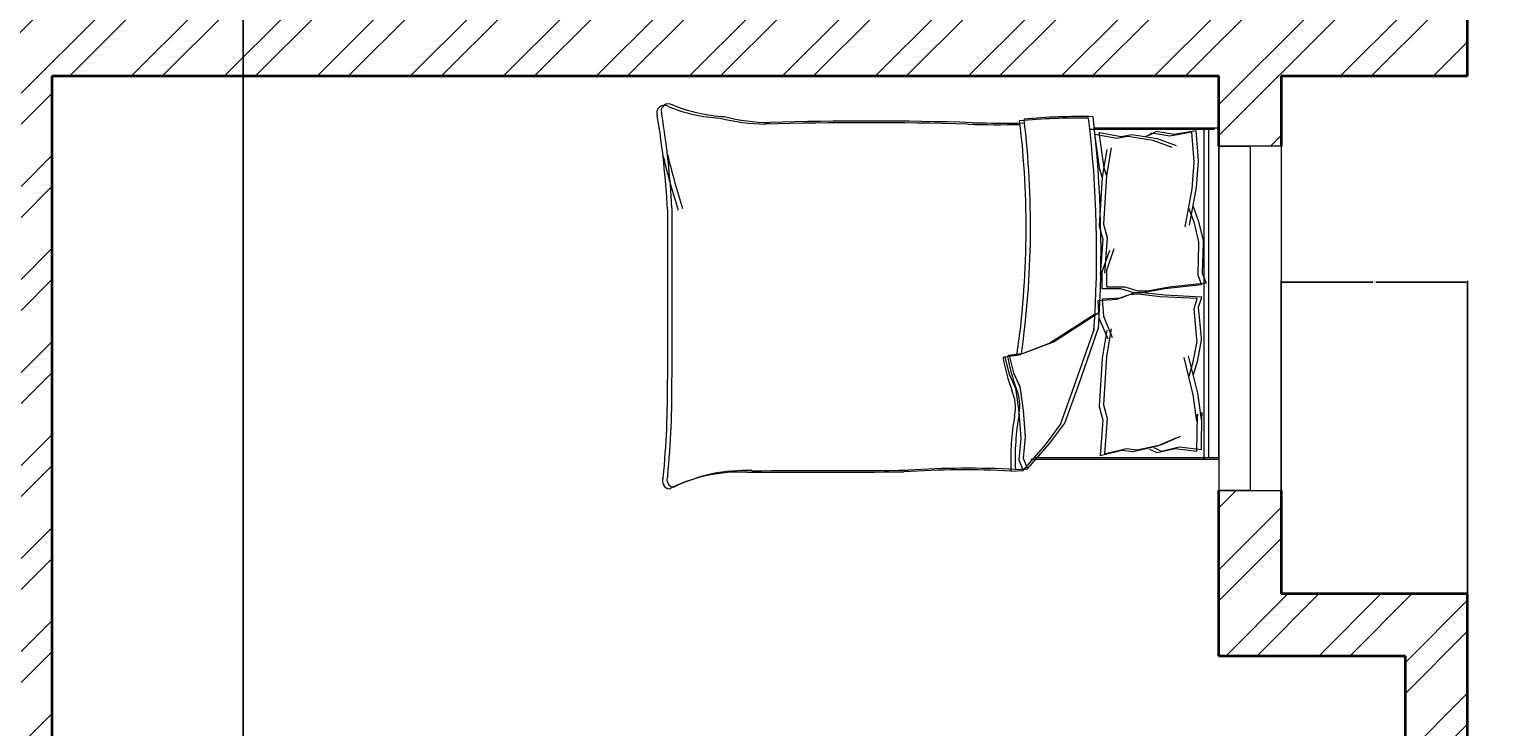
# Model space of a CAD drawing. Units: inches. Extents: x 1513 to 2170, y 1240 to 2288.
# Tile 5 of 10: x 1834 to 2045, y 1700 to 1801. Entities that reach past the tile are written whole.
import ezdxf

# ---------------------------------------------------------------- set-up
doc = ezdxf.new("R2010")
doc.units = ezdxf.units.IN
for name, color, linetype, lineweight in [('A-ANNO-DIMS', 2, 'Continuous', 18), ('A-FURN', 8, 'Continuous', 18), ('A-GLAZ', 4, 'Continuous', 18), ('A-WALL', 7, 'Continuous', 35), ('A-WALL-PATT', 252, 'Continuous', 13)]:
    doc.layers.add(name, color=color, linetype=linetype, lineweight=lineweight)
doc.styles.get("Standard").update_dxf_attribs({"font": 'arial.ttf'})
doc.dimstyles.get("Standard").update_dxf_attribs({"dimtxt": 0.18, "dimasz": 0.18, "dimexe": 0.18, "dimexo": 0.0625, "dimgap": 0.09, "dimtad": 0, "dimtih": 1, "dimtoh": 1, "dimdec": 4, "dimzin": 0, "dimdsep": 46, "dimtxsty": 'Standard', "dimcen": 0.09, "dimadec": 0, "dimazin": 0, "dimtfac": 1, "dimtdec": 4, "dimtofl": 0, "dimtmove": 0, "dimatfit": 3, "dimfxl": 1, "dimtolj": 1, "dimtzin": 0, "dimarcsym": 0})

# ---------------------------------------------------------------- blocks, each defined once
blk = doc.blocks.new('BED-DOUBLE')
for p, q in [((28.38, 53.1), (25.13, 49.39)), ((28.38, 53.1), (25.13, 49.39)), ((29.49, 52.95), (27.74, 52.87, 3.87)), ((29.49, 52.95), (27.74, 52.87, 3.87)), ((30.13, 53.18), (28.38, 53.1, 3.87)), ((30.13, 53.18), (28.38, 53.1, 3.87)), ((29, 51.56), (28.38, 53.1)), ((29, 51.56), (28.38, 53.1)), ((0, 51.27), (26.61, 51.27)), ((0, 51.27), (26.61, 51.27)), ((0.64, 51.49), (27.25, 51.49)), ((0.64, 51.49), (27.25, 51.49)), ((1.53, 3.48), (1.53, 51.27)), ((1.53, 3.48), (1.53, 51.27)), ((2.17, 3.7), (2.17, 51.49)), ((2.17, 3.7), (2.17, 51.49)), ((17.21, 50.93), (14.07, 50.15)), ((17.21, 50.93), (14.07, 50.15)), ((16.8, 45.8), (17.21, 50.93)), ((16.8, 45.8), (17.21, 50.93)), ((27.74, 52.87), (24.49, 49.16)), ((27.74, 52.87), (24.49, 49.16)), ((28.36, 51.33), (27.74, 52.87)), ((28.36, 51.33), (27.74, 52.87)), ((28.05, 48.23), (28.36, 51.33)), ((28.05, 48.23), (28.36, 51.33)), ((28.69, 48.46), (29, 51.56)), ((28.69, 48.46), (29, 51.56)), ((2.55, 50.11), (2.46, 44.71)), ((2.55, 50.11), (2.46, 44.71)), ((2.55, 50.11), (5.76, 49.73)), ((2.55, 50.11), (5.76, 49.73)), ((3.19, 50.34), (3.1, 44.94)), ((3.19, 50.34), (3.1, 44.94)), ((3.19, 50.34), (6.4, 49.96)), ((3.19, 50.34), (6.4, 49.96)), ((8.25, 49.31), (5.57, 48.13)), ((8.25, 49.31), (5.57, 48.13)), ((5.76, 49.73), (8.33, 50.33)), ((5.76, 49.73), (8.33, 50.33)), ((8.89, 49.54), (6.21, 48.36)), ((8.89, 49.54), (6.21, 48.36)), ((6.4, 49.96), (8.97, 50.56)), ((6.4, 49.96), (8.97, 50.56)), ((11.83, 50.11), (8.25, 49.31)), ((11.83, 50.11), (8.25, 49.31)), ((8.33, 50.33), (9.38, 49.82)), ((8.33, 50.33), (9.38, 49.82)), ((12.46, 50.34), (8.89, 49.54)), ((12.46, 50.34), (8.89, 49.54)), ((8.97, 50.56), (10.02, 50.04)), ((8.97, 50.56), (10.02, 50.04)), ((13.43, 49.92), (11.83, 50.11)), ((13.43, 49.92), (11.83, 50.11)), ((14.07, 50.15), (12.46, 50.34)), ((14.07, 50.15), (12.46, 50.34)), ((16.57, 50.7), (13.43, 49.92)), ((16.57, 50.7), (13.43, 49.92)), ((16.17, 45.57), (16.57, 50.7)), ((16.17, 45.57), (16.57, 50.7)), ((24.49, 49.16), (22.33, 46.22)), ((24.49, 49.16), (22.33, 46.22)), ((25.13, 49.39), (22.96, 46.45)), ((25.13, 49.39), (22.96, 46.45)), ((28.36, 44.36), (28.05, 48.23)), ((28.36, 44.36), (28.05, 48.23)), ((29, 44.59), (28.69, 48.46)), ((29, 44.59), (28.69, 48.46)), ((2.46, 44.71), (2.54, 45.71)), ((2.46, 44.71), (2.54, 45.71)), ((2.54, 45.71), (3.07, 41.92)), ((2.54, 45.71), (3.07, 41.92)), ((3.1, 44.94), (3.18, 45.94)), ((3.1, 44.94), (3.18, 45.94)), ((3.18, 45.94), (3.71, 42.14)), ((3.18, 45.94), (3.71, 42.14)), ((16.72, 43.61), (16.17, 45.57)), ((16.72, 43.61), (16.17, 45.57)), ((17.36, 43.84), (16.8, 45.8)), ((17.36, 43.84), (16.8, 45.8)), ((22.33, 46.22), (20.31, 40.65)), ((22.33, 46.22), (20.31, 40.65)), ((22.96, 46.45), (20.95, 40.87)), ((22.96, 46.45), (20.95, 40.87)), ((29.46, 41.18), (29, 44.59)), ((29.46, 41.18), (29, 44.59)), ((16.29, 36.6), (16.72, 43.61)), ((16.29, 36.6), (16.72, 43.61)), ((16.93, 36.83), (17.36, 43.84)), ((16.93, 36.83), (17.36, 43.84)), ((28.83, 40.96), (28.36, 44.36)), ((28.83, 40.95), (28.36, 44.36)), ((3.07, 41.92), (4.42, 36.5)), ((3.07, 41.92), (4.42, 36.5)), ((3.71, 42.14), (5.06, 36.72)), ((3.71, 42.14), (5.06, 36.72)), ((20.31, 40.65), (17.38, 32.31)), ((20.31, 40.65), (17.38, 32.31)), ((20.95, 40.87), (18.02, 32.54)), ((20.95, 40.87), (18.02, 32.54)), ((29.75, 38.94), (28.83, 40.96)), ((29.75, 38.94), (28.83, 40.95)), ((30.39, 39.17), (29.46, 41.18)), ((30.39, 39.17), (29.46, 41.18)), ((3.67, 39.2), (3.07, 37.14)), ((3.67, 39.2), (3.07, 37.14)), ((4.31, 39.43), (3.71, 37.36)), ((4.31, 39.43), (3.71, 37.36)), ((30.37, 36.46), (29.75, 38.94)), ((30.37, 36.46), (29.75, 38.94)), ((31.01, 36.69), (30.39, 39.17)), ((31.01, 36.69), (30.39, 39.17)), ((79.24, 15.06), (79.24, 39.68)), ((79.24, 15.06), (79.24, 39.68)), ((79.88, 15.29), (79.88, 39.91)), ((79.88, 15.29), (79.88, 39.91)), ((3.07, 37.14), (2.53, 34.21)), ((3.07, 37.14), (2.53, 34.21)), ((3.71, 37.36), (3.17, 34.43)), ((3.71, 37.36), (3.17, 34.43)), ((15.62, 32.57), (16.29, 36.6)), ((15.62, 32.57), (16.29, 36.6)), ((16.26, 32.79), (16.93, 36.83)), ((16.26, 32.79), (16.93, 36.83)), ((23.87, 34.45), (28.36, 36.15)), ((23.87, 34.45), (28.36, 36.15)), ((24.51, 34.68), (29, 36.38)), ((24.51, 34.68), (29, 36.38)), ((28.36, 36.15), (30.37, 36.46)), ((28.36, 36.15), (30.37, 36.46)), ((29, 36.38), (31.01, 36.69)), ((29, 36.38), (31.01, 36.69)), ((2.53, 34.21), (2.55, 33.88)), ((2.53, 34.21), (2.55, 33.88)), ((2.55, 33.88), (2.98, 29.46)), ((2.55, 33.88), (2.98, 29.46)), ((3.17, 34.43), (3.19, 34.11)), ((3.17, 34.43), (3.19, 34.11)), ((3.19, 34.11), (3.61, 29.69)), ((3.19, 34.11), (3.61, 29.68)), ((17.38, 30.98), (16.09, 34.05)), ((17.38, 30.98), (16.09, 34.05)), ((17.38, 30.26), (23.87, 34.45)), ((17.38, 30.26), (23.87, 34.45)), ((18.02, 30.49), (24.51, 34.68)), ((18.02, 30.49), (24.51, 34.68)), ((16.74, 30.75), (15.45, 33.82)), ((16.74, 30.75), (15.45, 33.82)), ((3.61, 29.69), (3.13, 28.21)), ((3.61, 29.68), (3.13, 28.21)), ((16.89, 28.3), (16.74, 30.75)), ((16.89, 28.3), (16.74, 30.75)), ((17.53, 28.53), (17.38, 30.98)), ((17.53, 28.53), (17.38, 30.98)), ((2.98, 29.46), (2.49, 27.98)), ((2.98, 29.46), (2.49, 27.98)), ((2.49, 27.98), (7.86, 27.73)), ((2.49, 27.98), (7.86, 27.73)), ((3.13, 28.21), (8.5, 27.96)), ((3.13, 28.21), (8.5, 27.96)), ((7.86, 27.73), (11.07, 27.36)), ((7.86, 27.73), (11.07, 27.36)), ((8.5, 27.96), (11.71, 27.58)), ((8.5, 27.96), (11.71, 27.58)), ((11.71, 27.58), (13.01, 27.67)), ((11.71, 27.58), (13.01, 27.67)), ((12.37, 27.44), (14.21, 28.13)), ((12.37, 27.44), (14.21, 28.13)), ((13.01, 27.67), (14.85, 28.36)), ((13.01, 27.67), (14.85, 28.36)), ((14.21, 28.13), (16.89, 28.3)), ((14.21, 28.13), (16.89, 28.3)), ((14.85, 28.36), (17.53, 28.53)), ((14.85, 28.36), (17.53, 28.53)), ((1.87, 25.98), (7.22, 26.56)), ((1.87, 25.98), (7.22, 26.56)), ((2.44, 24.54), (1.87, 25.98)), ((2.44, 24.54), (1.87, 25.98)), ((2.51, 26.21), (7.86, 26.79)), ((2.51, 26.21), (7.86, 26.79)), ((3.08, 24.77), (2.51, 26.21)), ((3.08, 24.77), (2.51, 26.21)), ((7.22, 26.56), (10.4, 27.14)), ((7.22, 26.56), (10.4, 27.14)), ((7.86, 26.79), (11.04, 27.37)), ((7.86, 26.79), (11.04, 27.37)), ((10.4, 27.14), (11.7, 27.14)), ((10.4, 27.14), (11.7, 27.14)), ((11.04, 27.37), (12.34, 27.37)), ((11.04, 27.37), (12.34, 27.37)), ((11.07, 27.36), (12.37, 27.44)), ((11.07, 27.36), (12.37, 27.44)), ((11.7, 27.14), (13.58, 26.56)), ((11.7, 27.14), (13.58, 26.56)), ((12.34, 27.37), (14.22, 26.79)), ((12.34, 27.37), (14.22, 26.79)), ((13.58, 26.56), (16.26, 26.56)), ((13.58, 26.56), (16.26, 26.56)), ((14.22, 26.79), (16.9, 26.79)), ((14.22, 26.79), (16.9, 26.79)), ((16.26, 26.56), (16.26, 24.1)), ((16.26, 26.56), (16.26, 24.1)), ((16.9, 26.79), (16.9, 24.33)), ((16.9, 26.79), (16.9, 24.33)), ((2.3, 20.09), (2.44, 24.54)), ((2.3, 20.09), (2.44, 24.54)), ((2.94, 20.32), (3.08, 24.77)), ((2.94, 20.32), (3.08, 24.77)), ((16.26, 24.1), (15.17, 20.96)), ((16.26, 24.1), (15.17, 20.96)), ((16.9, 24.33), (15.81, 21.19)), ((16.9, 24.33), (15.81, 21.19)), ((16.17, 19.39), (16.57, 24.52)), ((16.17, 19.38), (16.57, 24.52)), ((16.8, 19.61), (17.21, 24.75)), ((16.8, 19.61), (17.21, 24.74)), ((2.3, 19.77), (2.3, 20.09)), ((2.3, 19.77), (2.3, 20.09)), ((3.02, 16.88), (2.3, 19.77)), ((3.02, 16.88), (2.3, 19.77)), ((2.94, 20), (2.94, 20.32)), ((2.94, 20), (2.94, 20.32)), ((3.66, 17.11), (2.94, 20)), ((3.66, 17.11), (2.94, 20)), ((16.72, 17.42), (16.17, 19.39)), ((16.72, 17.42), (16.17, 19.38)), ((17.36, 17.65), (16.8, 19.61)), ((17.36, 17.65), (16.8, 19.61)), ((3.31, 12.11), (4.32, 17.6)), ((3.31, 12.11), (4.32, 17.6)), ((4.39, 15.08), (3.66, 17.11)), ((4.39, 15.08), (3.66, 17.11)), ((3.95, 12.34), (4.96, 17.83)), ((3.95, 12.34), (4.96, 17.83)), ((16.29, 10.41), (16.72, 17.42)), ((16.29, 10.41), (16.72, 17.42)), ((16.93, 10.64), (17.36, 17.65)), ((16.93, 10.64), (17.36, 17.65)), ((3.75, 14.86), (3.02, 16.88)), ((3.75, 14.86), (3.02, 16.88)), ((3.02, 8.29), (3.31, 12.11)), ((3.02, 8.29), (3.31, 12.11)), ((3.66, 8.51), (3.95, 12.34)), ((3.66, 8.51), (3.95, 12.34)), ((16.26, 6.61), (16.93, 10.64)), ((16.26, 6.61), (16.93, 10.64)), ((16.93, 10.64), (17.25, 9.51)), ((16.93, 10.64), (17.25, 9.51)), ((3.64, 8.41), (3.66, 8.51)), ((3.64, 8.41), (3.66, 8.51)), ((15.62, 6.38), (16.29, 10.41)), ((15.62, 6.38), (16.29, 10.41)), ((16.29, 10.41), (16.61, 9.28)), ((16.29, 10.41), (16.61, 9.28)), ((16.61, 9.28), (17.34, 4.18)), ((16.61, 9.28), (17.34, 4.18)), ((17.25, 9.51), (17.98, 4.41)), ((17.25, 9.51), (17.98, 4.41)), ((3.01, 8.18), (3.02, 8.29)), ((3.01, 8.18), (3.02, 8.29)), ((3.33, 3.9), (3.01, 8.18)), ((3.33, 3.9), (3.01, 8.18)), ((3.97, 4.13), (3.64, 8.41)), ((3.97, 4.13), (3.64, 8.41)), ((3.31, 3.9), (6.49, 4.47)), ((3.31, 3.9), (6.49, 4.47)), ((3.95, 4.12), (7.13, 4.7)), ((3.95, 4.12), (7.13, 4.7)), ((8.95, 5.05), (6.2, 6.06)), ((8.95, 5.05), (6.2, 6.06)), ((6.49, 4.47), (9.1, 4.04)), ((6.49, 4.47), (9.1, 4.04)), ((9.59, 5.28), (6.84, 6.29)), ((9.59, 5.28), (6.84, 6.29)), ((7.13, 4.7), (9.74, 4.27)), ((7.13, 4.7), (9.74, 4.27)), ((12.57, 4.47), (8.95, 5.05)), ((12.57, 4.47), (8.95, 5.05)), ((9.1, 4.04), (10.11, 4.62)), ((9.1, 4.04), (10.11, 4.62)), ((13.21, 4.7), (9.59, 5.28)), ((13.21, 4.7), (9.59, 5.28)), ((9.74, 4.27), (10.75, 4.85)), ((9.74, 4.27), (10.75, 4.85)), ((14.16, 4.76), (12.57, 4.47)), ((14.16, 4.76), (12.57, 4.47)), ((14.8, 4.99), (13.21, 4.7)), ((14.8, 4.99), (13.21, 4.7)), ((17.34, 4.18), (14.16, 4.76)), ((17.34, 4.18), (14.16, 4.76)), ((17.98, 4.41), (14.8, 4.99)), ((17.98, 4.41), (14.8, 4.99)), ((18.11, 3.48), (0, 3.48)), ((18.11, 3.48), (0, 3.48)), ((18.75, 3.7), (0.64, 3.7)), ((18.75, 3.7), (0.64, 3.7))]:
    blk.add_line(p, q)
for centre, radius, start, end in [((68.66, 76.16), 23.07, 267.4714, 296.4681), ((68.66, 76.16), 23.07, 267.4714, 296.4681), ((69.3, 76.39), 23.07, 267.4714, 296.4681), ((69.3, 76.39), 23.07, 267.4714, 296.4681), ((78.87, 54.41), 1.1, 332.6588, 86.02), ((78.87, 54.41), 1.1, 332.6588, 86.02), ((79.51, 54.64), 1.1, 332.6588, 86.02), ((79.51, 54.64), 1.1, 332.6588, 86.02), ((-6.66, 51.33), 36.18, 349.8763, 2.5657), ((-6.66, 51.33), 36.18, 349.8763, 2.5657), ((36.31, 182.27), 129.5, 266.9791, 273.8365), ((36.31, 182.27), 129.5, 266.9791, 273.8365), ((-6.02, 51.56), 36.18, 349.8763, 2.5657), ((-6.02, 51.56), 36.18, 349.8763, 2.5657), ((36.95, 182.5), 129.5, 266.9791, 273.8365), ((36.95, 182.5), 129.5, 266.9791, 273.8365), ((67.82, -4508.74), 4561.86, 90.00217, 90.28689), ((67.82, -4508.74), 4561.86, 90.00217, 90.28689), ((68.46, -4508.51), 4561.86, 90.00217, 90.28689), ((68.46, -4508.51), 4561.86, 90.00217, 90.28689), ((212.27, 41.15), 133.04, 174.4998, 180.6351), ((212.27, 41.15), 133.04, 174.4998, 180.6351), ((212.91, 41.38), 133.04, 174.4998, 180.6351), ((212.91, 41.38), 133.04, 174.4998, 180.6351), ((35.06, 43.74), 6.22, 168.6608, 203.7384), ((35.06, 43.74), 6.22, 168.6608, 203.7384), ((35.7, 43.97), 6.22, 168.6608, 203.7384), ((35.7, 43.97), 6.22, 168.6608, 203.7384), ((1.48, 31.15), 29.65, 10.6617, 19.8806), ((1.48, 31.15), 29.65, 10.6617, 19.8806), ((2.12, 31.38), 29.65, 10.6617, 19.8806), ((2.12, 31.38), 29.65, 10.6617, 19.8806), ((156.31, 17.76), 129.02, 171.7845, 186.9006), ((156.31, 17.76), 129.02, 171.7845, 186.9006), ((156.95, 17.99), 129.02, 171.7845, 186.9006), ((156.95, 17.98), 129.02, 171.7845, 186.9006), ((30.44, 36.64), 0.185, 250.2464, 1.1377), ((30.44, 36.64), 0.185, 250.2464, 1.1377), ((31.08, 36.87), 0.185, 250.2464, 1.1377), ((31.08, 36.87), 0.185, 250.2464, 1.1377), ((182.05, 21.36), 164.97, 176.0865, 186.7821), ((182.05, 21.36), 164.97, 176.0865, 186.7821), ((182.69, 21.59), 164.97, 176.0865, 186.7821), ((182.69, 21.59), 164.97, 176.0865, 186.7821), ((-23.72, -17.22), 106.46, 13.3832, 17.7053), ((-23.72, -17.22), 106.46, 13.3832, 17.7053), ((-23.08, -16.99), 106.46, 13.3832, 17.7053), ((-23.08, -16.99), 106.46, 13.3832, 17.7053), ((200.83, 21.43), 121.76, 182.9958, 189.4091), ((200.83, 21.43), 121.76, 182.9958, 189.4091), ((201.47, 21.66), 121.76, 182.9958, 189.4091), ((201.47, 21.66), 121.76, 182.9958, 189.4091), ((20.09, 85.16), 83.31, 268.7218, 275.604), ((20.09, 85.16), 83.31, 268.7218, 275.604), ((20.73, 85.39), 83.31, 268.7218, 275.604), ((20.73, 85.39), 83.31, 268.7218, 275.604), ((31.17, -167.31), 170.11, 88.4762, 91.0082), ((31.17, -167.31), 170.11, 88.4762, 91.0082), ((31.81, -167.08), 170.11, 88.4762, 91.0082), ((31.81, -167.08), 170.11, 88.4762, 91.0082), ((50.61, 484.82), 482.31, 268.2277, 271.7185), ((50.61, 484.82), 482.31, 268.2277, 271.7185), ((51.25, 485.05), 482.31, 268.2277, 271.7185), ((51.25, 485.05), 482.31, 268.2277, 271.7185), ((64.51, -26.9), 29.63, 76.0648, 88.9113), ((64.51, -26.9), 29.63, 76.0648, 88.9113), ((65.15, -26.67), 29.63, 76.0648, 88.9113), ((65.15, -26.67), 29.63, 76.0648, 88.9113), ((70.27, -21.66), 23.56, 67.9751, 86.652), ((70.27, -21.66), 23.56, 67.9751, 86.652), ((70.91, -21.43), 23.56, 67.9751, 86.652), ((70.91, -21.43), 23.56, 67.9751, 86.652), ((79.71, 1.09), 1.09, 236.1736, 23.4781), ((79.71, 1.09), 1.09, 236.1736, 23.4781), ((80.35, 1.32), 1.09, 236.1736, 23.4781), ((80.35, 1.32), 1.09, 236.1736, 23.4781)]:
    blk.add_arc(centre, radius, start, end)
blk = doc.blocks.new('*D26')
at = {"layer": 'A-ANNO-DIMS', "color": 0, "lineweight": -2, "transparency": 16777216}
for p, q in [((2014.91, 2214.48), (2087.18, 2214.48)), ((2087, 2214.3), (2087, 1802.16)), ((2087, 1389.66), (2087, 1801.8)), ((1937.43, 1389.48), (2087.18, 1389.48))]:
    blk.add_line(p, q, dxfattribs=at)
at = {"layer": 'A-ANNO-DIMS', "color": 0, "transparency": 16777216}
for points in [[(2086.97, 2214.3), (2087.03, 2214.3), (2087, 2214.48)], [(2086.97, 1389.66), (2087.03, 1389.66), (2087, 1389.48)]]:
    blk.add_solid(points, dxfattribs=at)
at = {"layer": 'Defpoints', "color": 0, "transparency": 16777216}
for p in [(2014.85, 2214.48), (2087, 2214.48), (1937.37, 1389.48)]:
    blk.add_point(p, dxfattribs=at)
at = {"layer": 'A-ANNO-DIMS', "color": 0, "transparency": 16777216, "insert": (2087, 1801.98), "char_height": 0.18, "attachment_point": 5}
blk.add_mtext('\\A1;825', dxfattribs=at)
blk = doc.blocks.new('*D28')
at = {"layer": 'A-ANNO-DIMS', "color": 0, "lineweight": -2, "transparency": 16777216}
for p, q in [((2014.85, 1719.54), (2014.85, 1764.81)), ((2015.03, 1764.63), (2028.13, 1764.63)), ((2041.67, 1764.63), (2028.57, 1764.63)), ((2041.85, 1719.54), (2041.85, 1764.81))]:
    blk.add_line(p, q, dxfattribs=at)
at = {"layer": 'A-ANNO-DIMS', "color": 0, "transparency": 16777216}
for points in [[(2015.03, 1764.66), (2015.03, 1764.6), (2014.85, 1764.63)], [(2041.67, 1764.66), (2041.67, 1764.6), (2041.85, 1764.63)]]:
    blk.add_solid(points, dxfattribs=at)
at = {"layer": 'Defpoints', "color": 0, "transparency": 16777216}
for p in [(2041.85, 1764.63), (2014.85, 1719.48), (2041.85, 1719.48)]:
    blk.add_point(p, dxfattribs=at)
at = {"layer": 'A-ANNO-DIMS', "color": 0, "transparency": 16777216, "insert": (2028.35, 1764.63), "char_height": 0.18, "attachment_point": 5}
blk.add_mtext('\\A1;27', dxfattribs=at)
blk = doc.blocks.new('*D36')
at = {"layer": 'A-ANNO-DIMS', "color": 0, "lineweight": -2, "transparency": 16777216}
for p, q in [((1829.49, 1887.42), (1829.49, 1344.15)), ((1864.51, 1887.42), (1864.51, 1344.15)), ((1829.67, 1344.33), (1846.61, 1344.33)), ((1864.33, 1344.33), (1847.39, 1344.33))]:
    blk.add_line(p, q, dxfattribs=at)
at = {"layer": 'A-ANNO-DIMS', "color": 0, "transparency": 16777216}
for points in [[(1829.67, 1344.36), (1829.67, 1344.3), (1829.49, 1344.33)], [(1864.33, 1344.36), (1864.33, 1344.3), (1864.51, 1344.33)]]:
    blk.add_solid(points, dxfattribs=at)
at = {"layer": 'Defpoints', "color": 0, "transparency": 16777216}
for p in [(1829.49, 1887.48), (1864.51, 1887.48), (1864.51, 1344.33)]:
    blk.add_point(p, dxfattribs=at)
at = {"layer": 'A-ANNO-DIMS', "color": 0, "transparency": 16777216, "insert": (1847, 1344.33), "char_height": 0.18, "attachment_point": 5}
blk.add_mtext('\\A1;35.02', dxfattribs=at)

msp = doc.modelspace()

# ---------------------------------------------------------------- hatches: boundary and pattern name
at = {"layer": 'A-WALL-PATT'}
h = msp.add_hatch(dxfattribs=at)
h.set_pattern_fill('ANSI32', color=256)
h.paths.add_polyline_path([(2041.852, 1719.48), (2014.852, 1719.48), (2014.852, 1734.444), (2005.852, 1734.444), (2005.852, 1710.48), (2032.852, 1710.48), (2032.852, 1663.98), (1976.619, 1663.98), (1976.619, 1659.48), (2005.852, 1659.48), (2005.852, 1626.27), (2014.852, 1626.27), (2014.852, 1659.48), (2041.852, 1659.48)])
h.paths.add_polyline_path([(1954.521, 1663.98), (1875.357, 1663.98), (1875.357, 1659.48), (1945.852, 1659.48), (1945.852, 1546.98), (1950.352, 1546.98), (2005.852, 1546.98), (2005.852, 1422.48), (1985.47, 1422.48), (1985.47, 1413.48), (2014.852, 1413.48), (2014.852, 1602.27), (2005.852, 1602.27), (2005.852, 1551.48), (1950.352, 1551.48), (1950.352, 1659.48), (1954.521, 1659.48)])
h.paths.add_polyline_path([(1949.47, 1422.48), (1937.366, 1422.48), (1937.366, 1413.48), (1949.47, 1413.48)], flags=0)
h.paths.add_polyline_path([(1937.366, 1422.48), (1908.866, 1422.48), (1908.866, 1546.98), (1805.486, 1546.98), (1805.486, 1542.48), (1904.366, 1542.48), (1904.366, 1451.2), (1897.222, 1451.2), (1897.222, 1442.2), (1904.366, 1442.2), (1904.366, 1422.48), (1904.366, 1413.48), (1904.366, 1389.48), (1908.866, 1389.48), (1908.866, 1413.48), (1932.866, 1413.48), (1932.866, 1389.48), (1937.366, 1389.48)])
h.paths.add_polyline_path([(1830.254, 1442.2), (1844.144, 1442.2), (1844.144, 1451.2), (1830.254, 1451.2), (1821.254, 1451.2), (1821.254, 1422.48), (1766.366, 1422.48), (1766.366, 1542.48), (1770.265, 1542.48), (1770.265, 1546.98), (1758.774, 1546.98), (1758.774, 1544.73), (1758.774, 1542.48), (1761.866, 1542.48), (1761.866, 1389.48), (1779.454, 1389.48), (1779.454, 1398.48), (1770.866, 1398.48), (1770.866, 1413.48), (1830.254, 1413.48)])
h.paths.add_polyline_path([(1686.156, 1451.2), (1677.156, 1451.2), (1677.156, 1422.48), (1623.866, 1422.48), (1623.866, 1460.073), (1614.866, 1460.073), (1614.866, 1413.48), (1686.156, 1413.48)])
h.paths.add_polyline_path([(1761.866, 1422.48), (1686.156, 1422.48), (1686.156, 1413.48), (1761.866, 1413.48)])
h.paths.add_polyline_path([(1623.866, 1542.48), (1688.266, 1542.48), (1688.266, 1544.73), (1688.266, 1546.98), (1623.866, 1546.98), (1623.866, 1560.442), (1614.866, 1560.442), (1614.866, 1520.073), (1619.366, 1520.073), (1623.866, 1520.073)])
h.paths.add_polyline_path([(1623.866, 1600.98), (1715.366, 1600.98), (1715.366, 1546.98), (1711.055, 1546.98), (1711.055, 1542.48), (1719.866, 1542.48), (1726.867, 1542.48), (1726.867, 1544.73), (1726.867, 1546.98), (1719.866, 1546.98), (1719.866, 1600.98), (1719.866, 1608.301), (1717.616, 1608.301), (1715.366, 1608.301), (1715.366, 1605.48), (1623.866, 1605.48), (1623.866, 1620.254), (1614.866, 1620.254), (1614.866, 1584.442), (1623.866, 1584.442)])
h.paths.add_polyline_path([(1623.866, 1659.48), (1715.366, 1659.48), (1715.366, 1629.2), (1719.866, 1629.2), (1719.866, 1659.48), (1767.866, 1659.48), (1767.866, 1629.2), (1772.366, 1629.2), (1772.366, 1663.98), (1578.866, 1663.98), (1578.866, 1661.73), (1578.866, 1659.48), (1578.866, 1635.48), (1583.366, 1635.48), (1583.366, 1654.98), (1614.866, 1654.98), (1614.866, 1644.254), (1619.366, 1644.254), (1623.866, 1644.254)])
h.paths.add_polyline_path([(1788.587, 1798.98), (1788.587, 1803.48), (1623.866, 1803.48), (1623.866, 1887.48), (1829.49, 1887.48), (1829.49, 1891.98), (1829.49, 1896.48), (1748.366, 1896.48), (1743.866, 1896.48), (1623.866, 1896.48), (1623.866, 1904.333), (1619.366, 1904.333), (1614.866, 1904.333), (1614.866, 1896.48), (1578.866, 1896.48), (1578.866, 1887.48), (1614.866, 1887.48), (1614.866, 1803.48), (1578.866, 1803.48), (1578.866, 1794.48), (1626.866, 1794.48), (1788.587, 1794.48)])
h.paths.add_polyline_path([(1635.866, 1794.48), (1626.866, 1794.48), (1626.866, 1763.627), (1631.366, 1763.627), (1635.866, 1763.627)])
h.paths.add_polyline_path([(1635.866, 1703.627), (1626.866, 1703.627), (1626.866, 1663.98), (1635.866, 1663.98)])
h.paths.add_polyline_path([(1587.866, 2016.48), (1614.866, 2016.48), (1623.866, 2016.48), (1707.767, 2016.48), (1707.767, 2018.73), (1707.767, 2020.98), (1706.366, 2020.98), (1706.366, 2025.944), (1701.866, 2025.944), (1701.866, 2020.98), (1623.866, 2020.98), (1623.866, 2045.903), (1614.866, 2045.903), (1614.866, 2025.48), (1583.366, 2025.48), (1583.366, 2040.48), (1578.866, 2040.48), (1578.866, 2016.48), (1578.866, 1956.48), (1614.866, 1956.48), (1614.866, 1946.333), (1623.866, 1946.333), (1623.866, 1965.48), (1587.866, 1965.48)])
h.paths.add_polyline_path([(1748.366, 2016.48), (1748.366, 2025.48), (1743.866, 2025.48), (1739.366, 2025.48), (1739.366, 2020.98), (1738.09, 2020.98), (1738.09, 2016.48), (1743.866, 2016.48), (1743.866, 1896.48), (1748.366, 1896.48)])
h.paths.add_polyline_path([(1746.736, 2085.48), (1623.866, 2085.48), (1623.866, 2205.48), (1657.136, 2205.48), (1657.136, 2214.48), (1614.866, 2214.48), (1614.866, 2069.903), (1623.866, 2069.903), (1623.866, 2080.98), (1683.866, 2080.98), (1701.866, 2080.98), (1701.866, 2046.743), (1706.366, 2046.743), (1706.366, 2080.98), (1746.736, 2080.98)])
h = msp.add_hatch(dxfattribs=at)
h.set_pattern_fill('ANSI32', color=256)
h.paths.add_polyline_path([(1744.852, 2209.98), (1762.042, 2209.98), (1762.042, 2214.48), (1715.345, 2214.48), (1715.345, 2205.48), (1735.852, 2205.48), (1735.852, 2161.98), (1733.253, 2161.98), (1719.866, 2161.98), (1719.866, 2112.429), (1724.366, 2112.429), (1724.366, 2152.98), (1762.042, 2152.98), (1870.852, 2152.98), (1870.852, 2080.98), (1875.352, 2080.98), (1878.245, 2080.98), (1878.245, 2083.23), (1878.245, 2085.48), (1875.352, 2085.48), (1875.352, 2173.929), (1881.628, 2173.929), (1881.628, 2178.429), (1881.628, 2182.929), (1875.352, 2182.929), (1875.352, 2214.48), (1858.335, 2214.48), (1858.335, 2209.98), (1866.352, 2209.98), (1866.352, 2161.98), (1762.042, 2161.98), (1744.852, 2161.98)])
h.paths.add_polyline_path([(2014.852, 2214.48), (1944.011, 2214.48), (1944.011, 2182.929), (1938.347, 2182.929), (1938.347, 2173.929), (1953.011, 2173.929), (1953.011, 2182.929), (1953.011, 2205.48), (2005.852, 2205.48), (2005.852, 2085.48), (1955.061, 2085.48), (1955.061, 2080.98), (2005.852, 2080.98), (2005.852, 2068.903), (2014.852, 2068.903)])
h.paths.add_polyline_path([(2014.852, 2044.903), (2005.852, 2044.903), (2005.852, 2020.98), (1926.352, 2020.98), (1926.352, 2080.98), (1930.882, 2080.98), (1930.882, 2083.23), (1930.882, 2085.48), (1921.852, 2085.48), (1915.536, 2085.48), (1915.536, 2083.23), (1915.536, 2080.98), (1921.852, 2080.98), (1921.852, 2020.98), (1916.378, 2020.98), (1916.378, 2018.73), (1916.378, 2016.48), (2005.852, 2016.48), (2005.852, 2009.442), (2014.852, 2009.442), (2014.852, 2016.48), (2029.852, 2016.48), (2041.852, 2016.48), (2041.852, 2040.48), (2037.352, 2040.48), (2037.352, 2036.595), (2037.352, 2020.98), (2014.852, 2020.98)])
h.paths.add_polyline_path([(2041.852, 1956.48), (2014.852, 1956.48), (2014.852, 1963.797), (2005.852, 1963.797), (2005.852, 1947.48), (2032.852, 1947.48), (2032.852, 1896.48), (1978.852, 1896.48), (1978.852, 1891.98), (1978.852, 1887.48), (2005.852, 1887.48), (2005.852, 1862.401), (2014.852, 1862.401), (2014.852, 1887.48), (2037.352, 1887.48), (2037.352, 1863.48), (2041.852, 1863.48), (2041.852, 1887.48), (2041.852, 1896.48)], flags=17)
h.paths.add_polyline_path([(1885.852, 1896.48), (1885.852, 1920.48), (1878.866, 1920.48), (1878.866, 2016.48), (1881.925, 2016.48), (1881.925, 2018.73), (1881.925, 2020.98), (1874.366, 2020.98), (1874.366, 1896.48), (1864.508, 1896.48), (1864.508, 1887.48), (1876.852, 1887.48), (1876.852, 1855.773), (1885.852, 1855.773), (1885.852, 1868.947), (1942.852, 1868.947), (1942.852, 1803.48), (1885.852, 1803.48), (1885.852, 1817.861), (1876.852, 1817.861), (1876.852, 1803.48), (1825.976, 1803.48), (1825.976, 1798.98), (1825.976, 1794.48), (1832.366, 1794.48), (1832.366, 1663.98), (1832.366, 1659.48), (1841.939, 1659.48), (1841.939, 1661.73), (1841.939, 1663.98), (1836.866, 1663.98), (1836.866, 1794.48), (1992.866, 1794.48), (2005.852, 1794.48), (2005.852, 1784.304), (2010.352, 1784.304), (2014.852, 1784.304), (2014.852, 1794.48), (2041.852, 1794.48), (2041.852, 1803.48), (2014.852, 1803.48), (2014.852, 1838.401), (2005.852, 1838.401), (2005.852, 1803.48), (1951.852, 1803.48), (1951.852, 1887.48), (1956.114, 1887.48), (1956.114, 1891.98), (1956.114, 1896.48), (1951.852, 1896.48), (1951.852, 1920.48), (1947.352, 1920.48), (1947.352, 1896.48), (1942.852, 1896.48), (1942.852, 1877.947), (1885.852, 1877.947)])

# ---------------------------------------------------------------- linework, layer by layer
at = {"layer": 'A-FURN'}
for p, q in [((2005.852, 1739.176), (2005.852, 1786.967)), ((2005.852, 1738.948), (2005.213, 1738.948))]:
    msp.add_line(p, q, dxfattribs=at)
at = {"layer": 'A-GLAZ'}
for p, q in [((2014.852, 1784.304), (2005.852, 1784.304)), ((2005.852, 1784.304), (2010.352, 1784.304)), ((2005.852, 1784.304), (2005.852, 1734.444)), ((2010.352, 1784.304), (2010.352, 1734.444)), ((2014.852, 1784.304), (2014.852, 1734.444)), ((2010.352, 1734.444), (2005.852, 1734.444)), ((2005.852, 1734.444), (2014.852, 1734.444))]:
    msp.add_line(p, q, dxfattribs=at)
at = {"layer": 'A-WALL'}
for p, q in [((2041.852, 1794.48), (2041.852, 1803.48)), ((1836.866, 1663.98), (1836.866, 1794.48)), ((1836.866, 1794.48), (1992.866, 1794.48)), ((1836.866, 1794.48), (2005.852, 1794.48)), ((2005.852, 1784.304), (2005.852, 1794.48)), ((2014.852, 1794.48), (2014.852, 1784.304)), ((2014.852, 1794.48), (2041.852, 1794.48)), ((2005.852, 1710.48), (2005.852, 1734.444)), ((2014.852, 1734.444), (2014.852, 1719.48)), ((2041.852, 1719.48), (2014.852, 1719.48)), ((2041.852, 1659.48), (2041.852, 1719.48)), ((2032.852, 1710.48), (2005.852, 1710.48)), ((2032.852, 1663.98), (2032.852, 1710.48))]:
    msp.add_line(p, q, dxfattribs=at)

# ---------------------------------------------------------------- block references
at = {"layer": 'A-FURN', "rotation": 180}
msp.add_blockref('BED-DOUBLE', (2005.848, 1790.443), dxfattribs=at)

# ---------------------------------------------------------------- dimensions: what is measured, and where the dimension line sits
at = {"layer": 'A-ANNO-DIMS'}
for base, p1, p2, angle, picture, middle in [((2087.002, 2214.48), (1937.366, 1389.48), (2014.852, 2214.48), 90, '*D26', (2087.002, 1801.98)), ((2041.852, 1764.63), (2014.852, 1719.48), (2041.852, 1719.48), 0, '*D28', (2028.352, 1764.63))]:
    dim = msp.add_linear_dim(base=base, p1=p1, p2=p2, angle=angle, dimstyle='Standard', override={"dimdec": 0, "dimlfac": 1, "dimrnd": 0, "dimzin": 0, "dimdsep": 46, "dimlunit": 2}, dxfattribs=at)
    dim.commit()
    dim.dimension.update_dxf_attribs({"geometry": picture, "text_midpoint": middle})
dim = msp.add_linear_dim(base=(1864.508, 1344.33), p1=(1829.49, 1887.48), p2=(1864.508, 1887.48), dimstyle='Standard', override={"dimdec": 2, "dimlfac": 1, "dimrnd": 0, "dimzin": 0, "dimdsep": 46, "dimlunit": 2}, dxfattribs=at)
dim.commit()
dim.dimension.update_dxf_attribs({"geometry": '*D36', "text_midpoint": (1846.999, 1344.33)})

doc.saveas('drawing.dxf')
